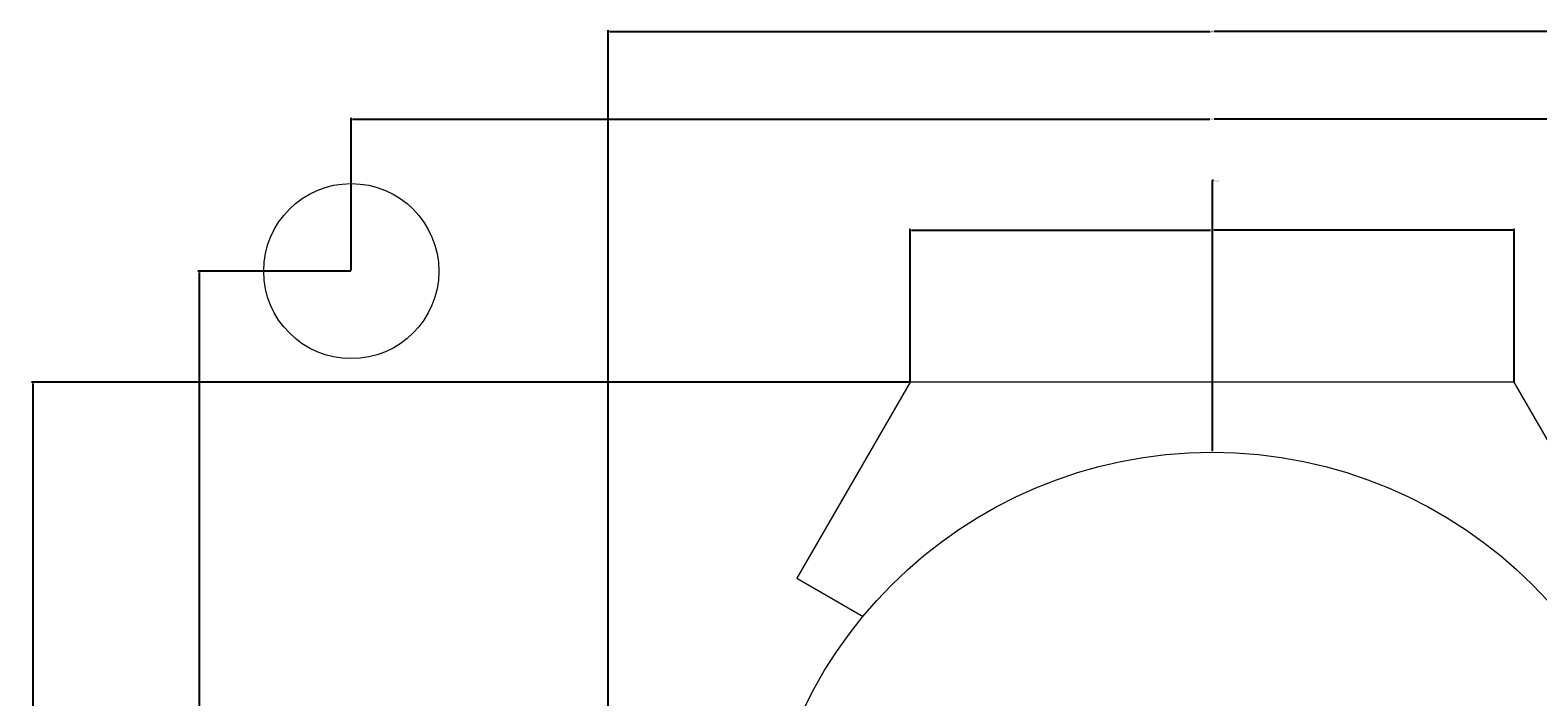
# Model space of a CAD drawing. Units: inches. Extents: x 1095 to 1408, y -20 to 240.
# Tile 5 of 8: x 1095 to 1294, y 152 to 240. Entities that reach past the tile are written whole.
import ezdxf

# ---------------------------------------------------------------- set-up
doc = ezdxf.new("R2010")
doc.units = ezdxf.units.IN
doc.header["$MEASUREMENT"] = 0
doc.layers.add('M-CONS', color=8, linetype='Continuous', lineweight=18)
doc.layers.add('M-DIMS', color=2, linetype='Continuous', lineweight=18)
doc.styles.get("Standard").update_dxf_attribs({"font": 'arial.ttf'})
doc.dimstyles.get("Standard").update_dxf_attribs({"dimtxt": 0.18, "dimasz": 0.18, "dimexe": 0.18, "dimexo": 0.0625, "dimgap": 0.09, "dimtad": 0, "dimtih": 1, "dimtoh": 1, "dimdec": 4, "dimzin": 0, "dimdsep": 46, "dimtxsty": 'Standard', "dimcen": 0.09, "dimadec": 0, "dimazin": 0, "dimtfac": 1, "dimtdec": 4, "dimtofl": 0, "dimtmove": 0, "dimatfit": 3, "dimfxl": 1, "dimtolj": 1, "dimtzin": 0, "dimarcsym": 0})

# ---------------------------------------------------------------- blocks, each defined once
blk = doc.blocks.new('*D5')
at = {"layer": 'Defpoints', "color": 0, "transparency": 16777216}
for p in [(1365.18, 228.15), (1137.18, 208), (1365.18, 208)]:
    blk.add_point(p, dxfattribs=at)
at = {"layer": 'M-DIMS', "color": 0, "lineweight": -2, "transparency": 16777216}
for p, q in [((1137.18, 208.06), (1137.18, 228.33)), ((1137.36, 228.15), (1250.89, 228.15)), ((1365, 228.15), (1251.47, 228.15)), ((1365.18, 208.06), (1365.18, 228.33))]:
    blk.add_line(p, q, dxfattribs=at)
at = {"layer": 'M-DIMS', "color": 0, "transparency": 16777216}
for points in [[(1137.36, 228.18), (1137.36, 228.12), (1137.18, 228.15)], [(1365, 228.18), (1365, 228.12), (1365.18, 228.15)]]:
    blk.add_solid(points, dxfattribs=at)
at = {"layer": 'M-DIMS', "color": 0, "transparency": 16777216, "insert": (1251.18, 228.15), "char_height": 0.18, "attachment_point": 5}
blk.add_mtext('\\A1;228', dxfattribs=at)
blk = doc.blocks.new('*D6')
at = {"layer": 'Defpoints', "color": 0, "transparency": 16777216}
for p in [(1117.03, 208), (1137.18, 208), (1137.18, 40)]:
    blk.add_point(p, dxfattribs=at)
at = {"layer": 'M-DIMS', "color": 0, "lineweight": -2, "transparency": 16777216}
for p, q in [((1137.12, 208), (1116.85, 208)), ((1117.03, 207.82), (1117.03, 124.18)), ((1117.03, 40.18), (1117.03, 123.82)), ((1137.12, 40), (1116.85, 40))]:
    blk.add_line(p, q, dxfattribs=at)
at = {"layer": 'M-DIMS', "color": 0, "transparency": 16777216}
for points in [[(1117, 207.82), (1117.06, 207.82), (1117.03, 208)], [(1117, 40.18), (1117.06, 40.18), (1117.03, 40)]]:
    blk.add_solid(points, dxfattribs=at)
at = {"layer": 'M-DIMS', "color": 0, "transparency": 16777216, "insert": (1117.03, 124), "char_height": 0.18, "attachment_point": 5}
blk.add_mtext('\\A1;168', dxfattribs=at)
blk = doc.blocks.new('*D9')
at = {"layer": 'Defpoints', "color": 0, "transparency": 16777216}
for p in [(1331.18, 239.75), (1171.18, 124), (1331.18, 124)]:
    blk.add_point(p, dxfattribs=at)
at = {"layer": 'M-DIMS', "color": 0, "lineweight": -2, "transparency": 16777216}
for p, q in [((1171.18, 124.06), (1171.18, 239.93)), ((1171.36, 239.75), (1250.9, 239.75)), ((1331, 239.75), (1251.46, 239.75)), ((1331.18, 124.06), (1331.18, 239.93))]:
    blk.add_line(p, q, dxfattribs=at)
at = {"layer": 'M-DIMS', "color": 0, "transparency": 16777216}
for points in [[(1171.36, 239.78), (1171.36, 239.72), (1171.18, 239.75)], [(1331, 239.78), (1331, 239.72), (1331.18, 239.75)]]:
    blk.add_solid(points, dxfattribs=at)
at = {"layer": 'M-DIMS', "color": 0, "transparency": 16777216, "insert": (1251.18, 239.75), "char_height": 0.18, "attachment_point": 5}
blk.add_mtext('\\A1;160', dxfattribs=at)
blk = doc.blocks.new('*D10')
at = {"layer": 'Defpoints', "color": 0, "transparency": 16777216}
for p in [(1095.03, 193.28), (1211.18, 193.28), (1211.18, 54.72)]:
    blk.add_point(p, dxfattribs=at)
at = {"layer": 'M-DIMS', "color": 0, "lineweight": -2, "transparency": 16777216}
for p, q in [((1211.12, 193.28), (1094.85, 193.28)), ((1095.03, 193.1), (1095.03, 124.18)), ((1095.03, 54.9), (1095.03, 123.82)), ((1211.12, 54.72), (1094.85, 54.72))]:
    blk.add_line(p, q, dxfattribs=at)
at = {"layer": 'M-DIMS', "color": 0, "transparency": 16777216}
for points in [[(1095, 193.1), (1095.06, 193.1), (1095.03, 193.28)], [(1095, 54.9), (1095.06, 54.9), (1095.03, 54.72)]]:
    blk.add_solid(points, dxfattribs=at)
at = {"layer": 'M-DIMS', "color": 0, "transparency": 16777216, "insert": (1095.03, 124), "char_height": 0.18, "attachment_point": 5}
blk.add_mtext('\\A1;138.56', dxfattribs=at)
blk = doc.blocks.new('*D11')
at = {"layer": 'Defpoints', "color": 0, "transparency": 16777216}
for p in [(1291.18, 213.43), (1211.18, 193.28), (1291.18, 193.28)]:
    blk.add_point(p, dxfattribs=at)
at = {"layer": 'M-DIMS', "color": 0, "lineweight": -2, "transparency": 16777216}
for p, q in [((1211.18, 193.34), (1211.18, 213.61)), ((1211.36, 213.43), (1250.96, 213.43)), ((1291, 213.43), (1251.4, 213.43)), ((1291.18, 193.34), (1291.18, 213.61))]:
    blk.add_line(p, q, dxfattribs=at)
at = {"layer": 'M-DIMS', "color": 0, "transparency": 16777216}
for points in [[(1211.36, 213.46), (1211.36, 213.4), (1211.18, 213.43)], [(1291, 213.46), (1291, 213.4), (1291.18, 213.43)]]:
    blk.add_solid(points, dxfattribs=at)
at = {"layer": 'M-DIMS', "color": 0, "transparency": 16777216, "insert": (1251.18, 213.43), "char_height": 0.18, "attachment_point": 5}
blk.add_mtext('\\A1;80', dxfattribs=at)
blk = doc.blocks.new('*D18')
at = {"layer": 'Defpoints', "color": 0, "transparency": 16777216}
for p in [(1251.18, 184), (1251.18, 64)]:
    blk.add_point(p, dxfattribs=at)
at = {"layer": 'M-DIMS', "color": 0, "lineweight": -2, "transparency": 16777216}
for p, q in [((1251.36, 220), (1251.18, 220)), ((1251.18, 220), (1251.18, 184.18)), ((1251.09, 124), (1251.27, 124)), ((1251.18, 123.91), (1251.18, 124.09))]:
    blk.add_line(p, q, dxfattribs=at)
at = {"layer": 'M-DIMS', "color": 0, "transparency": 16777216}
blk.add_solid([(1251.15, 184.18), (1251.21, 184.18), (1251.18, 184)], dxfattribs=at)
at = {"layer": 'M-DIMS', "color": 0, "transparency": 16777216, "insert": (1251.75, 220), "char_height": 0.18, "attachment_point": 5}
blk.add_mtext('\\A1;∅120', dxfattribs=at)

msp = doc.modelspace()

# ---------------------------------------------------------------- linework, layer by layer
at = {"layer": 'M-CONS', "elevation": 377.783}
msp.add_lwpolyline([(1297.418, 162.241), (1306.184, 167.301), (1291.184, 193.282), (1211.184, 193.282), (1196.184, 167.301), (1204.949, 162.241)], dxfattribs=at)
at = {"layer": 'M-CONS'}
for centre, radius in [((1137.184, 208, 397.783), 11.6), ((1251.184, 124, 377.783), 60)]:
    msp.add_circle(centre, radius, dxfattribs=at)

# ---------------------------------------------------------------- dimensions: what is measured, and where the dimension line sits
at = {"layer": 'M-DIMS'}
for base, p1, p2, picture, middle in [((1331.184, 239.75), (1171.184, 124), (1331.184, 124), '*D9', (1251.184, 239.75)), ((1365.184, 228.15), (1137.184, 208), (1365.184, 208), '*D5', (1251.184, 228.15)), ((1291.184, 213.432), (1211.184, 193.282), (1291.184, 193.282), '*D11', (1251.184, 213.432))]:
    dim = msp.add_linear_dim(base=base, p1=p1, p2=p2, dimstyle='Standard', override={"dimdec": 0, "dimlfac": 1, "dimrnd": 0, "dimzin": 0, "dimdsep": 46, "dimlunit": 2}, dxfattribs=at)
    dim.commit()
    dim.dimension.update_dxf_attribs({"geometry": picture, "text_midpoint": middle})
dim = msp.add_diameter_dim_2p(p1=(1251.183, 64), p2=(1251.184, 184), dimstyle='Standard', override={"dimdec": 0, "dimlfac": 1, "dimrnd": 0, "dimzin": 0, "dimdsep": 46, "dimlunit": 2}, dxfattribs=at)
dim.commit()
dim.dimension.update_dxf_attribs({"geometry": '*D18', "text_midpoint": (1251.751, 220), "dimtype": 163})
for base, p1, p2, override, picture, middle in [((1117.034, 208), (1137.184, 40), (1137.184, 208), {"dimdec": 0, "dimlfac": 1, "dimrnd": 0, "dimzin": 0, "dimdsep": 46, "dimlunit": 2}, '*D6', (1117.034, 124)), ((1095.034, 193.282), (1211.184, 54.718), (1211.184, 193.282), {"dimdec": 2, "dimlfac": 1, "dimrnd": 0, "dimzin": 0, "dimdsep": 46, "dimlunit": 2}, '*D10', (1095.034, 124))]:
    dim = msp.add_linear_dim(base=base, p1=p1, p2=p2, angle=90, dimstyle='Standard', override=override, dxfattribs=at)
    dim.commit()
    dim.dimension.update_dxf_attribs({"geometry": picture, "text_midpoint": middle})

doc.saveas('drawing.dxf')
